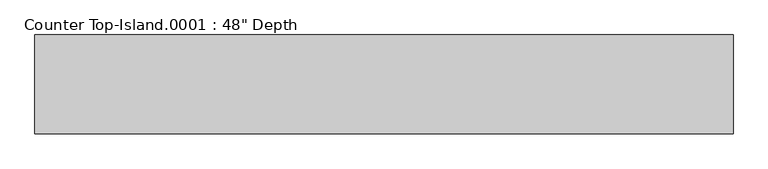
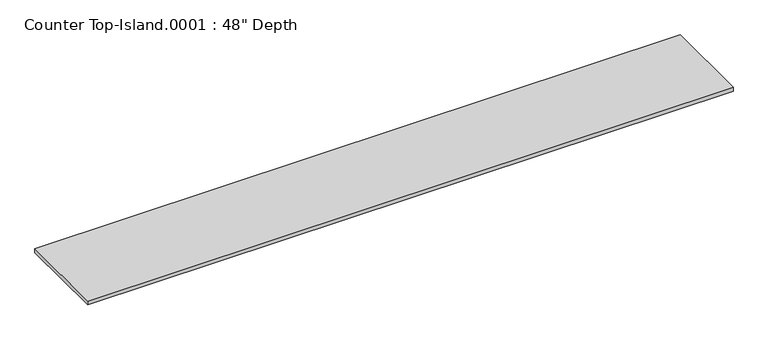
"""IFC4 building model written with IfcOpenShell, lengths in millimetres: furniture geometry."""

from ifc_helpers import new_model, si_unit, frame, origin, place, context, project, spatial, polyline, outline, extrude, source, transform, mapped, element, save


def furniture_b7a5125e(model_context):
    return source(origin(), model_context, "Body", "SweptSolid", [
        extrude(outline(polyline([(4819.3377049, 25.4), (4819.3377049, -825.5), (-1200.4622951, -825.5), (-1200.4622951, 25.4), (4819.3377049, 25.4)])), frame((0.0, 0.0, 571.5), z_axis=(0.0, 0.0, 1.0), x_axis=(1.0, 0.0, 0.0)), (0.0, 0.0, 1.0), 38.1),
    ])


if __name__ == "__main__":
    model = new_model("IFC4")
    model_context = context("Model", 3, world=origin())
    ifc_project = project(units=[si_unit("LENGTHUNIT", "METRE", prefix="MILLI")], contexts=[model_context])
    site = spatial("IfcSite", under=ifc_project)
    building = spatial("IfcBuilding", under=site)
    placement = place(None, origin())
    furniture_shape = furniture_b7a5125e(model_context)
    element("IfcFurniture", 1, ObjectType="Counter Top-Island.0001 : 48\" Depth", at=placement, inside=building, context=model_context, shape_type="MappedRepresentation", body=[
        mapped(furniture_shape, transform((0.0, 0.0, 0.0), x_axis=(1.0, 0.0, 0.0), y_axis=(0.0, 1.0, 0.0), z_axis=(0.0, 0.0, 1.0))),
    ])
    save(model, "model.ifc")

# Revit data of these elements
# Type "Counter Top-Island.0001 : 48\" Depth"
#   Assembly Code = "C1030400"
#   Counter Thickness = 0' - 1 1/2"
#   Depth [instance default] = 4' - 2"
#   Height = 2' - 0"
#   Length [instance default] = 8' - 0"
#   Counter Top Material = none
#   Default Elevation = 0
# Element 1 (IfcFurniture, "Counter Top-Island.0001 : 48\" Depth")
#   Depth = 2' - 9 1/2"
#   Length = 19' - 9"
#   Materials on its faces: "Counter Top"
# Materials
#   "Counter Top": class "Wood", colour RGB 226 177 128, transparency 0
